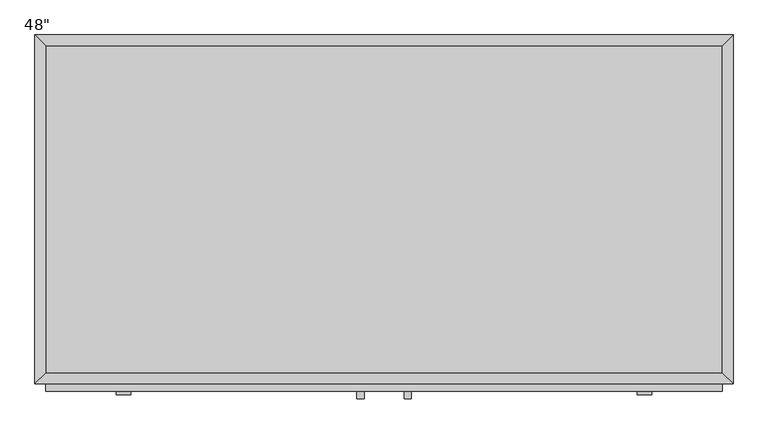
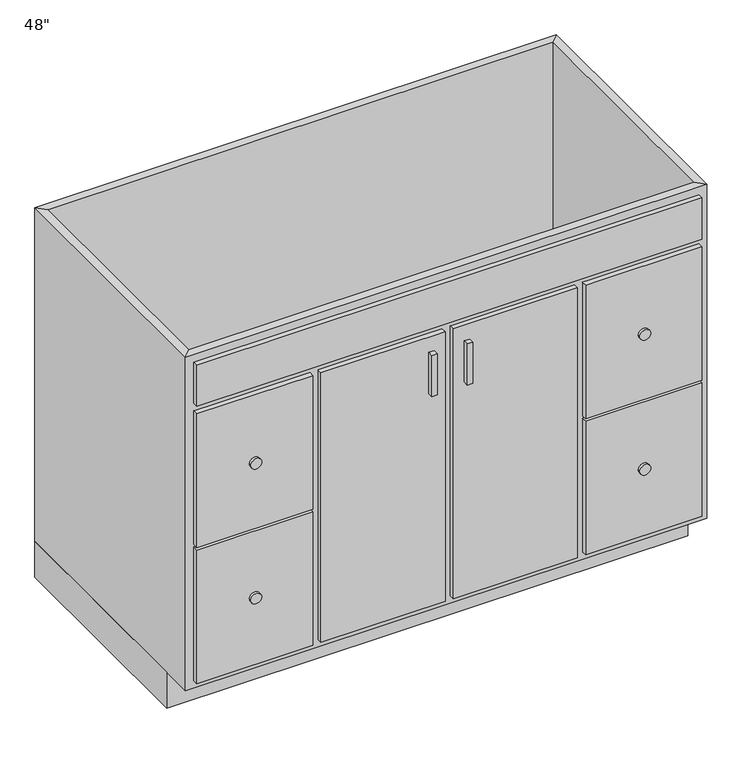
"""IFC4 building model written with IfcOpenShell, lengths in millimetres: furniture geometry."""

from ifc_helpers import new_model, si_unit, point, frame, frame_2d, origin, origin_with_axes, place, context, project, spatial, polyline, circle_curve, trimmed, segment, composite_curve, outline, extrude, faceted_brep, source, transform, mapped, element, save


def furniture_48488436(model_context):
    return source(origin(), model_context, "Body", "SolidModel", [
        extrude(outline(polyline([(700.44496, 0.0), (700.44496, -533.4), (-518.75504, -533.4), (-518.75504, 0.0), (700.44496, 0.0)])), origin_with_axes(), (0.0, 0.0, 1.0), 88.9),
        faceted_brep([(681.39496, -590.55, 914.4), (681.39496, -590.55, 88.9), (-499.70504, -590.55, 88.9), (-499.70504, -590.55, 914.4), (700.44496, -609.6, 914.4), (-518.75504, -609.6, 914.4), (700.44496, -609.6, 88.9), (-518.75504, -609.6, 88.9), (-499.70504, -19.05, 88.9), (-499.70504, -19.05, 914.4), (-518.75504, 0.0, 914.4), (-518.75504, 0.0, 88.9), (681.39496, -19.05, 88.9), (681.39496, -19.05, 914.4), (700.44496, 0.0, 914.4), (700.44496, 0.0, 88.9)], [[[0, 1, 2, 3]], [[4, 0, 3, 5]], [[6, 4, 5, 7]], [[1, 6, 7, 2]], [[3, 2, 8, 9]], [[5, 3, 9, 10]], [[7, 5, 10, 11]], [[2, 7, 11, 8]], [[9, 8, 12, 13]], [[10, 9, 13, 14]], [[11, 10, 14, 15]], [[8, 11, 15, 12]], [[13, 12, 1, 0]], [[14, 13, 0, 4]], [[15, 14, 4, 6]], [[12, 15, 6, 1]]]),
        extrude(outline(polyline([(681.39496, -19.05), (681.39496, -590.55), (-499.70504, -590.55), (-499.70504, -19.05), (681.39496, -19.05)])), frame((0.0, 0.0, 88.9), z_axis=(0.0, 0.0, 1.0), x_axis=(1.0, 0.0, 0.0)), (0.0, 0.0, 1.0), 19.05),
        extrude(outline(composite_curve([segment(trimmed(circle_curve(frame_2d((274.6375, 545.66371)), 12.7), [point((274.6375, 532.96371))], [point((274.6375, 558.36371))], False, "CARTESIAN"), True, "CONTINUOUS"), segment(trimmed(circle_curve(frame_2d((274.6375, 545.66371)), 12.7), [point((274.6375, 558.36371))], [point((274.6375, 532.96371))], False, "CARTESIAN"), True, "CONTINUOUS")], self_intersect=False)), frame((0.0, -628.65, 0.0), z_axis=(0.0, 1.0, 0.0), x_axis=(0.0, 0.0, 1.0)), (0.0, 0.0, 1.0), 6.35),
        extrude(outline(composite_curve([segment(trimmed(circle_curve(frame_2d((608.0125, 545.66371)), 12.7), [point((608.0125, 532.96371))], [point((608.0125, 558.36371))], False, "CARTESIAN"), True, "CONTINUOUS"), segment(trimmed(circle_curve(frame_2d((608.0125, 545.66371)), 12.7), [point((608.0125, 558.36371))], [point((608.0125, 532.96371))], False, "CARTESIAN"), True, "CONTINUOUS")], self_intersect=False)), frame((0.0, -628.65, 0.0), z_axis=(0.0, 1.0, 0.0), x_axis=(0.0, 0.0, 1.0)), (0.0, 0.0, 1.0), 6.35),
        extrude(outline(composite_curve([segment(trimmed(circle_curve(frame_2d((608.0125, -363.97379)), 12.7), [point((608.0125, -376.67379))], [point((608.0125, -351.27379))], False, "CARTESIAN"), True, "CONTINUOUS"), segment(trimmed(circle_curve(frame_2d((608.0125, -363.97379)), 12.7), [point((608.0125, -351.27379))], [point((608.0125, -376.67379))], False, "CARTESIAN"), True, "CONTINUOUS")], self_intersect=False)), frame((0.0, -628.65, 0.0), z_axis=(0.0, 1.0, 0.0), x_axis=(0.0, 0.0, 1.0)), (0.0, 0.0, 1.0), 6.35),
        extrude(outline(composite_curve([segment(trimmed(circle_curve(frame_2d((274.6375, -363.97379)), 12.7), [point((274.6375, -376.67379))], [point((274.6375, -351.27379))], False, "CARTESIAN"), True, "CONTINUOUS"), segment(trimmed(circle_curve(frame_2d((274.6375, -363.97379)), 12.7), [point((274.6375, -351.27379))], [point((274.6375, -376.67379))], False, "CARTESIAN"), True, "CONTINUOUS")], self_intersect=False)), frame((0.0, -628.65, 0.0), z_axis=(0.0, 1.0, 0.0), x_axis=(0.0, 0.0, 1.0)), (0.0, 0.0, 1.0), 6.35),
        extrude(outline(polyline([(55.91996, -635.0), (43.21996, -635.0), (43.21996, -622.3), (55.91996, -622.3), (55.91996, -635.0)])), frame((0.0, 0.0, 635.0), z_axis=(0.0, 0.0, 1.0), x_axis=(1.0, 0.0, 0.0)), (0.0, 0.0, 1.0), 101.6),
        extrude(outline(polyline([(138.46996, -635.0), (125.76996, -635.0), (125.76996, -622.3), (138.46996, -622.3), (138.46996, -635.0)])), frame((0.0, 0.0, 635.0), z_axis=(0.0, 0.0, 1.0), x_axis=(1.0, 0.0, 0.0)), (0.0, 0.0, 1.0), 101.6),
        extrude(outline(polyline([(681.39496, -622.3), (-499.70504, -622.3), (-499.70504, -609.6), (681.39496, -609.6), (681.39496, -622.3)])), frame((0.0, 0.0, 793.75), z_axis=(0.0, 0.0, 1.0), x_axis=(1.0, 0.0, 0.0)), (0.0, 0.0, 1.0), 101.6),
        extrude(outline(polyline([(681.39496, -622.3), (409.93246, -622.3), (409.93246, -609.6), (681.39496, -609.6), (681.39496, -622.3)])), frame((0.0, 0.0, 444.5), z_axis=(0.0, 0.0, 1.0), x_axis=(1.0, 0.0, 0.0)), (0.0, 0.0, 1.0), 330.2),
        extrude(outline(polyline([(681.39496, -622.3), (409.93246, -622.3), (409.93246, -609.6), (681.39496, -609.6), (681.39496, -622.3)])), frame((0.0, 0.0, 107.95), z_axis=(0.0, 0.0, 1.0), x_axis=(1.0, 0.0, 0.0)), (0.0, 0.0, 1.0), 330.2),
        extrude(outline(polyline([(-228.24254, -622.3), (-499.70504, -622.3), (-499.70504, -609.6), (-228.24254, -609.6), (-228.24254, -622.3)])), frame((0.0, 0.0, 444.5), z_axis=(0.0, 0.0, 1.0), x_axis=(1.0, 0.0, 0.0)), (0.0, 0.0, 1.0), 330.2),
        extrude(outline(polyline([(-228.24254, -622.3), (-499.70504, -622.3), (-499.70504, -609.6), (-228.24254, -609.6), (-228.24254, -622.3)])), frame((0.0, 0.0, 107.95), z_axis=(0.0, 0.0, 1.0), x_axis=(1.0, 0.0, 0.0)), (0.0, 0.0, 1.0), 330.2),
        extrude(outline(polyline([(81.31996, -622.3), (-209.19254, -622.3), (-209.19254, -609.6), (81.31996, -609.6), (81.31996, -622.3)])), frame((0.0, 0.0, 107.95), z_axis=(0.0, 0.0, 1.0), x_axis=(1.0, 0.0, 0.0)), (0.0, 0.0, 1.0), 666.75),
        extrude(outline(polyline([(390.88246, -622.3), (100.36996, -622.3), (100.36996, -609.6), (390.88246, -609.6), (390.88246, -622.3)])), frame((0.0, 0.0, 107.95), z_axis=(0.0, 0.0, 1.0), x_axis=(1.0, 0.0, 0.0)), (0.0, 0.0, 1.0), 666.75),
    ])


if __name__ == "__main__":
    model = new_model("IFC4")
    model_context = context("Model", 3, world=origin())
    ifc_project = project(units=[si_unit("LENGTHUNIT", "METRE", prefix="MILLI")], contexts=[model_context])
    site = spatial("IfcSite", under=ifc_project)
    building = spatial("IfcBuilding", under=site)
    placement = place(None, origin())
    furniture_shape = furniture_48488436(model_context)
    element("IfcFurniture", 1, ObjectType="48\"", at=placement, inside=building, context=model_context, shape_type="MappedRepresentation", body=[
        mapped(furniture_shape, transform((0.0, 0.0, 0.0), x_axis=(1.0, 0.0, 0.0), y_axis=(0.0, 1.0, 0.0), z_axis=(0.0, 0.0, 1.0))),
    ])
    save(model, "model.ifc")

# Revit data of these elements
# Type "48\""
#   Assembly Code = "C1030410"
#   Depth = 2' - 0"
#   Height = 3' - 0"
#   Toe Depth = 0' - 3"
#   Toe Height = 0' - 3 1/2"
#   Width = 4' - 0"
#   Cabinet Material = none
#   Door/Drawer Material = none
#   Handle Material = Cabinets - Handles
#   Default Elevation = 0
# Element 1 (IfcFurniture, "48\"")
#   Materials on its faces: "Cabinets", "Cabinets - Handles"
# Materials
#   "Cabinets - Handles": class "Metal", colour RGB 57 57 57, transparency 0
#   "Cabinets": colour RGB 249 249 249, transparency 0
